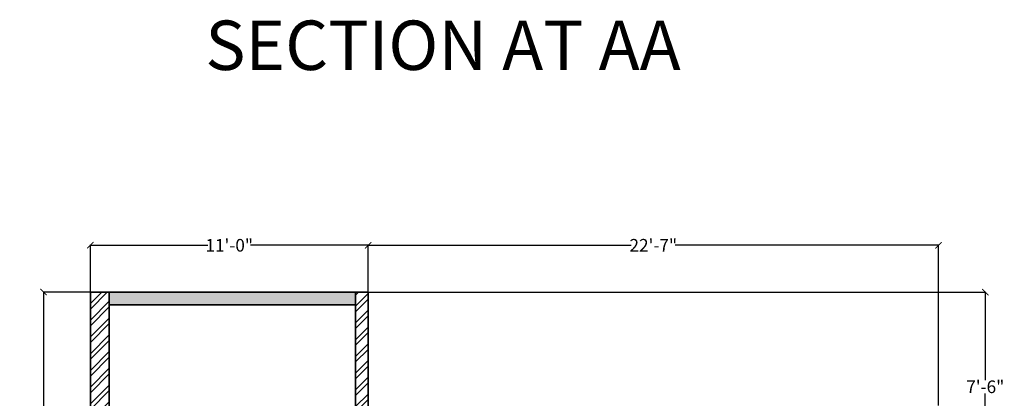
# Model space of a CAD drawing. Units: inches. Extents: x 2278 to 7495, y -71 to 1198.
# Tile 41 of 44: x 6954 to 7421, y 439 to 619. Entities that reach past the tile are written whole.
import ezdxf

# ---------------------------------------------------------------- set-up
doc = ezdxf.new("R2010")
doc.units = ezdxf.units.IN
doc.header["$MEASUREMENT"] = 0
for name, color, linetype, lineweight in [('A-ANNO-DIMS', 2, 'Continuous', 18), ('A-AREA-IDEN', 3, 'Continuous', 18), ('A-SECT', 7, 'Continuous', 35), ('A-SECT-PATT', 8, 'Continuous', 13)]:
    doc.layers.add(name, color=color, linetype=linetype, lineweight=lineweight)
doc.styles.get("Standard").update_dxf_attribs({"font": 'arial.ttf'})
doc.dimstyles.get("Standard").update_dxf_attribs({"dimtxt": 6, "dimasz": 3, "dimexe": 0.18, "dimexo": 0.0625, "dimgap": 0.09, "dimtad": 0, "dimtih": 1, "dimtoh": 1, "dimdec": 0, "dimzin": 0, "dimdsep": 46, "dimlunit": 3, "dimtxsty": 'Standard', "dimblk": 'ARCHTICK', "dimcen": 0.09, "dimadec": 0, "dimazin": 0, "dimtfac": 1, "dimtdec": 0, "dimtofl": 0, "dimtmove": 0, "dimatfit": 3, "dimfxl": 1, "dimtolj": 1, "dimtzin": 0, "dimarcsym": 0})

# ---------------------------------------------------------------- blocks, each defined once
blk = doc.blocks.new('_ArchTick')
at = {"color": 0, "linetype": 'ByBlock', "const_width": 0.15}
blk.add_lwpolyline([(-0.5, -0.5), (0.5, 0.5)], dxfattribs=at)
blk = doc.blocks.new('*D113')
at = {"layer": 'A-ANNO-DIMS', "color": 0, "lineweight": -2, "transparency": 16777216}
for p, q in [((7119.18, 489.83), (7412.55, 489.83)), ((7412.37, 489.83), (7412.37, 447.99)), ((7412.37, 399.83), (7412.37, 441.68)), ((7119.18, 399.83), (7412.55, 399.83))]:
    blk.add_line(p, q, dxfattribs=at)
at = {"layer": 'Defpoints', "color": 0, "transparency": 16777216}
for p in [(7119.12, 489.83), (7412.37, 489.83), (7119.12, 399.83)]:
    blk.add_point(p, dxfattribs=at)
at = {"layer": 'A-ANNO-DIMS', "color": 0, "lineweight": -2, "transparency": 16777216, "xscale": 3, "yscale": 3, "zscale": 3}
for p, rotation in [((7412.37, 489.83), 90), ((7412.37, 399.83), 270)]:
    blk.add_blockref('_ArchTick', p, dxfattribs=dict(at, rotation=rotation))
at = {"layer": 'A-ANNO-DIMS', "color": 0, "transparency": 16777216, "insert": (7412.37, 444.83), "char_height": 6, "attachment_point": 5}
blk.add_mtext('\\A1;7\'-6"', dxfattribs=at)
blk = doc.blocks.new('*D114')
at = {"layer": 'A-ANNO-DIMS', "color": 0, "lineweight": -2, "transparency": 16777216}
for p, q in [((6987.05, 489.83), (6964.69, 489.83)), ((6964.87, 489.83), (6964.87, 324.99)), ((6964.87, 153.83), (6964.87, 318.68)), ((6987.05, 153.83), (6964.69, 153.83))]:
    blk.add_line(p, q, dxfattribs=at)
at = {"layer": 'Defpoints', "color": 0, "transparency": 16777216}
for p in [(6964.87, 489.83), (6987.12, 489.83), (6987.12, 153.83)]:
    blk.add_point(p, dxfattribs=at)
at = {"layer": 'A-ANNO-DIMS', "color": 0, "lineweight": -2, "transparency": 16777216, "xscale": 3, "yscale": 3, "zscale": 3}
for p, rotation in [((6964.87, 489.83), 90), ((6964.87, 153.83), 270)]:
    blk.add_blockref('_ArchTick', p, dxfattribs=dict(at, rotation=rotation))
at = {"layer": 'A-ANNO-DIMS', "color": 0, "transparency": 16777216, "insert": (6964.87, 321.83), "char_height": 6, "attachment_point": 5}
blk.add_mtext('\\A1;28\'-0"', dxfattribs=at)
blk = doc.blocks.new('*D121')
at = {"layer": 'A-ANNO-DIMS', "color": 0, "lineweight": -2, "transparency": 16777216}
for p, q in [((6987.12, 489.9), (6987.12, 512.26)), ((6987.12, 512.08), (7043, 512.08)), ((7119.12, 512.08), (7063.23, 512.08)), ((7119.12, 489.9), (7119.12, 512.26))]:
    blk.add_line(p, q, dxfattribs=at)
at = {"layer": 'Defpoints', "color": 0, "transparency": 16777216}
for p in [(7119.12, 512.08), (6987.12, 489.83), (7119.12, 489.83)]:
    blk.add_point(p, dxfattribs=at)
at = {"layer": 'A-ANNO-DIMS', "color": 0, "lineweight": -2, "transparency": 16777216, "xscale": 3, "yscale": 3, "zscale": 3, "rotation": 180}
blk.add_blockref('_ArchTick', (6987.12, 512.08), dxfattribs=at)
at = {"layer": 'A-ANNO-DIMS', "color": 0, "lineweight": -2, "transparency": 16777216, "xscale": 3, "yscale": 3, "zscale": 3}
blk.add_blockref('_ArchTick', (7119.12, 512.08), dxfattribs=at)
at = {"layer": 'A-ANNO-DIMS', "color": 0, "transparency": 16777216, "insert": (7053.12, 512.08), "char_height": 6, "attachment_point": 5}
blk.add_mtext('\\A1;11\'-0"', dxfattribs=at)
blk = doc.blocks.new('*D122')
at = {"layer": 'A-ANNO-DIMS', "color": 0, "lineweight": -2, "transparency": 16777216}
for p, q in [((7119.12, 489.9), (7119.12, 512.26)), ((7119.12, 512.08), (7244.17, 512.08)), ((7390.11, 512.08), (7265.06, 512.08)), ((7390.11, 435.95), (7390.11, 512.26))]:
    blk.add_line(p, q, dxfattribs=at)
at = {"layer": 'Defpoints', "color": 0, "transparency": 16777216}
for p in [(7390.11, 512.08), (7119.12, 489.83), (7390.11, 435.89)]:
    blk.add_point(p, dxfattribs=at)
at = {"layer": 'A-ANNO-DIMS', "color": 0, "lineweight": -2, "transparency": 16777216, "xscale": 3, "yscale": 3, "zscale": 3, "rotation": 180}
blk.add_blockref('_ArchTick', (7119.12, 512.08), dxfattribs=at)
at = {"layer": 'A-ANNO-DIMS', "color": 0, "lineweight": -2, "transparency": 16777216, "xscale": 3, "yscale": 3, "zscale": 3}
blk.add_blockref('_ArchTick', (7390.11, 512.08), dxfattribs=at)
at = {"layer": 'A-ANNO-DIMS', "color": 0, "transparency": 16777216, "insert": (7254.61, 512.08), "char_height": 6, "attachment_point": 5}
blk.add_mtext('\\A1;22\'-7"', dxfattribs=at)

msp = doc.modelspace()

# ---------------------------------------------------------------- hatches: boundary and pattern name
at = {"layer": 'A-SECT-PATT', "transparency": 33554687}
h = msp.add_hatch(dxfattribs=at)
h.set_pattern_fill('ANSI32', color=256, scale=15)
h.set_pattern_definition([(45, (0, 155.58), (-3.9774756, 3.9774756), []), (45, (2.6517, 155.58), (-3.9774756, 3.9774756), [])])
h.paths.add_polyline_path([(6996.12, 489.83), (6987.12, 489.83), (6987.12, 153.83), (6996.12, 153.83)])
h.paths.add_polyline_path([(7390.12, 399.83), (7381.12, 399.83), (7381.12, 153.83), (7390.12, 153.83)])
h.paths.add_polyline_path([(7119.12, 483.83), (7119.12, 489.83), (7113.12, 489.83), (7113.12, 399.83), (7119.12, 399.83)])
h = msp.add_hatch(dxfattribs=at)
h.set_pattern_fill('GOST_GROUND', color=256, scale=0.1)
h.set_pattern_definition([(45, (0, 155.5801), (1.41421356, 0), [2]), (45, (0.3, 155.5801), (1.41421356, 0), [2]), (45, (0.6, 155.5801), (1.41421356, 0), [2])])
h.paths.add_polyline_path([(7113.12, 489.83), (6996.12, 489.83), (6996.12, 483.83), (7113.12, 483.83)])

# ---------------------------------------------------------------- linework, layer by layer
at = {"layer": 'A-SECT'}
for p, q in [((6987.12, 153.83), (6987.12, 489.83)), ((7113.12, 489.83), (6987.12, 489.83)), ((6996.12, 153.83), (6996.12, 489.83)), ((7113.12, 399.83), (7113.12, 489.83)), ((7119.12, 489.83), (7113.12, 489.83)), ((7119.12, 483.83), (7119.12, 489.83)), ((7119.12, 489.83), (7119.12, 374.25)), ((7113.12, 483.83), (6996.12, 483.83)), ((7119.12, 399.83), (7119.12, 483.83))]:
    msp.add_line(p, q, dxfattribs=at)

# ---------------------------------------------------------------- texts
at = {"layer": 'A-AREA-IDEN'}
msp.add_text('SECTION AT AA', height=23.4811, dxfattribs=at).set_placement((7041.75, 595.41))

# ---------------------------------------------------------------- dimensions: what is measured, and where the dimension line sits
at = {"layer": 'A-ANNO-DIMS'}
for base, p1, p2, picture, middle in [((7119.12, 512.08), (6987.12, 489.83), (7119.12, 489.83), '*D121', (7053.12, 512.08)), ((7390.11, 512.08), (7119.12, 489.83), (7390.11, 435.89), '*D122', (7254.61, 512.08))]:
    dim = msp.add_linear_dim(base=base, p1=p1, p2=p2, dimstyle='Standard', override={"dimdec": 1, "dimlfac": 1, "dimrnd": 0, "dimzin": 1, "dimdsep": 46, "dimlunit": 4, "dimfrac": 2}, dxfattribs=at)
    dim.commit()
    dim.dimension.update_dxf_attribs({"geometry": picture, "text_midpoint": middle})
for base, p1, p2, picture, middle in [((6964.87, 489.83), (6987.12, 153.83), (6987.12, 489.83), '*D114', (6964.87, 321.83)), ((7412.37, 489.83), (7119.12, 399.83), (7119.12, 489.83), '*D113', (7412.37, 444.83))]:
    dim = msp.add_linear_dim(base=base, p1=p1, p2=p2, angle=90, dimstyle='Standard', override={"dimdec": 1, "dimlfac": 1, "dimrnd": 0, "dimzin": 1, "dimdsep": 46, "dimlunit": 4, "dimfrac": 2}, dxfattribs=at)
    dim.commit()
    dim.dimension.update_dxf_attribs({"geometry": picture, "text_midpoint": middle})

doc.saveas('drawing.dxf')
